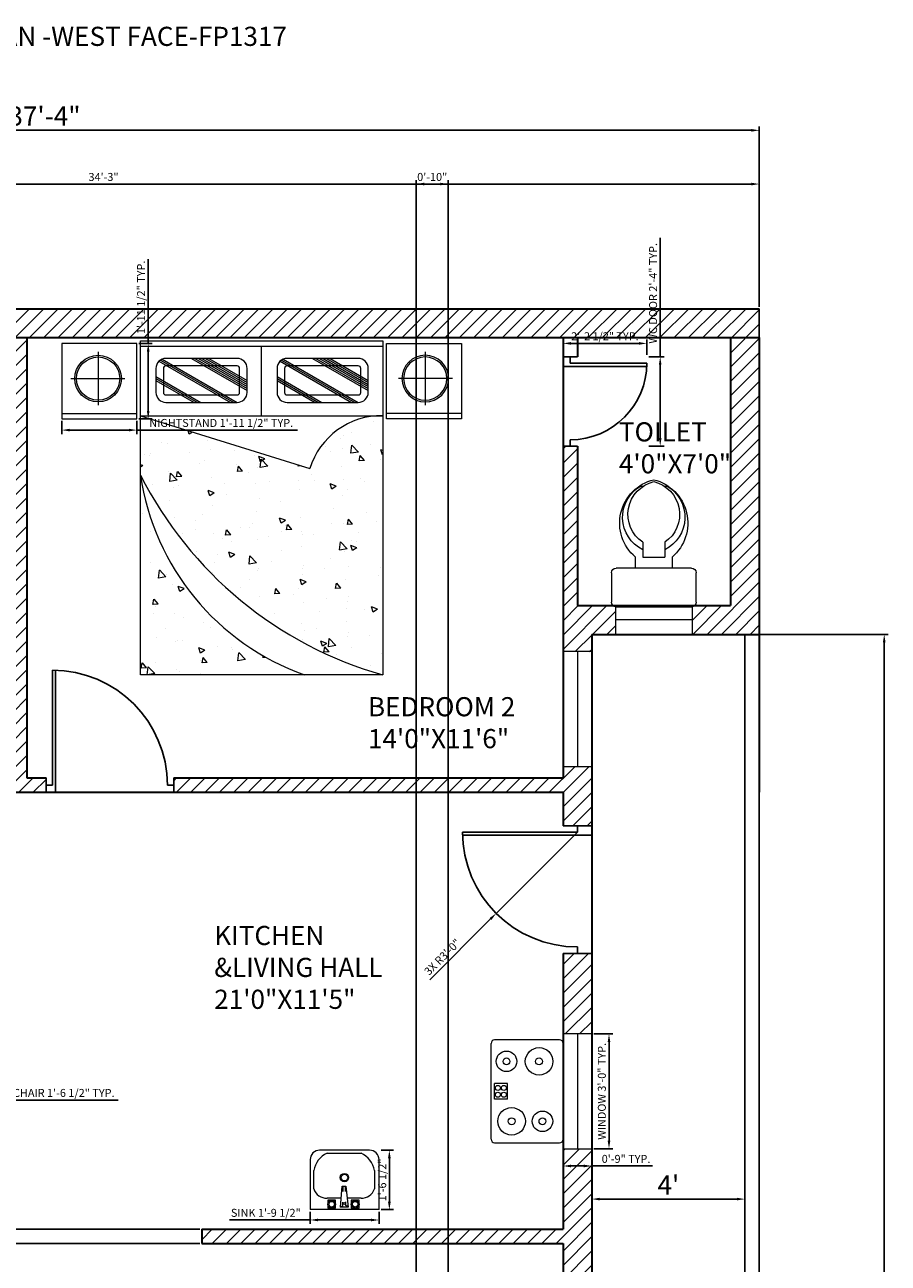
# Model space of a CAD drawing. Units: inches. Extents: x 3618 to 4156, y 1271 to 2023.
# Tile 5 of 5: x 3886 to 4156, y 1635 to 2023. Entities that reach past the tile are written whole.
import ezdxf

# ---------------------------------------------------------------- set-up
doc = ezdxf.new("R2010")
doc.units = ezdxf.units.IN
for name, color, linetype, lineweight in [('A-ANNO-DIMS', 2, 'Continuous', 18), ('A-ANNO-TITL', 7, 'Continuous', 25), ('A-AREA-IDEN', 7, 'Continuous', 18), ('A-DOOR', 4, 'Continuous', 25), ('A-EQPM', 8, 'Continuous', 18), ('A-FLOR-FIXT', 9, 'Continuous', 18), ('A-FURN', 8, 'Continuous', 18), ('A-FURN-PATT', 9, 'Continuous', 13), ('A-GLAZ', 4, 'Continuous', 18), ('A-WALL', 7, 'Continuous', 35), ('A-WALL-PATT', 252, 'Continuous', 13), ('C-PROP', 7, 'Continuous', 25)]:
    doc.layers.add(name, color=color, linetype=linetype, lineweight=lineweight)
doc.styles.get("Standard").update_dxf_attribs({"font": 'arial.ttf'})
doc.dimstyles.new('ISO-25', dxfattribs={"dimtxt": 2.5, "dimasz": 2.5, "dimexe": 1.25, "dimexo": 0.625, "dimtad": 1, "dimdec": 0, "dimlunit": 3, "dimtxsty": 'Standard', "dimcen": 2.5, "dimadec": 0, "dimazin": 0, "dimtfac": 1, "dimtdec": 0, "dimtmove": 0, "dimatfit": 3, "dimfxl": 1, "dimarcsym": 0})

# ---------------------------------------------------------------- blocks, each defined once
blk = doc.blocks.new('*D1')
at = {"layer": 'A-ANNO-DIMS', "color": 0, "lineweight": -2, "transparency": 16777216}
for p, q in [((4063.19, 1642.81), (4063.19, 1656.03)), ((4065.69, 1654.78), (4108.69, 1654.78)), ((4111.19, 1642.81), (4111.19, 1656.03))]:
    blk.add_line(p, q, dxfattribs=at)
at = {"layer": 'A-ANNO-DIMS', "color": 0, "transparency": 16777216}
for points in [[(4065.69, 1655.2), (4065.69, 1654.37), (4063.19, 1654.78)], [(4108.69, 1655.2), (4108.69, 1654.37), (4111.19, 1654.78)]]:
    blk.add_solid(points, dxfattribs=at)
at = {"layer": 'Defpoints', "color": 0, "transparency": 16777216}
for p in [(4111.19, 1654.78), (4063.19, 1642.19), (4111.19, 1642.19)]:
    blk.add_point(p, dxfattribs=at)
at = {"layer": 'A-ANNO-DIMS', "color": 0, "transparency": 16777216, "insert": (4087.19, 1658.41), "char_height": 6, "attachment_point": 5}
blk.add_mtext("4'", dxfattribs=at)
blk = doc.blocks.new('*D4')
at = {"layer": 'A-ANNO-DIMS', "color": 0, "lineweight": -2, "transparency": 16777216}
for p, q in [((3667.69, 1934.44), (3667.69, 1991.05)), ((3670.19, 1989.8), (4113.19, 1989.8)), ((4115.69, 1934.44), (4115.69, 1991.05))]:
    blk.add_line(p, q, dxfattribs=at)
at = {"layer": 'A-ANNO-DIMS', "color": 0, "transparency": 16777216}
for points in [[(3670.19, 1990.21), (3670.19, 1989.38), (3667.69, 1989.8)], [(4113.19, 1990.21), (4113.19, 1989.38), (4115.69, 1989.8)]]:
    blk.add_solid(points, dxfattribs=at)
at = {"layer": 'Defpoints', "color": 0, "transparency": 16777216}
for p in [(4115.69, 1989.8), (3667.69, 1933.81), (4115.69, 1933.81)]:
    blk.add_point(p, dxfattribs=at)
at = {"layer": 'A-ANNO-DIMS', "color": 0, "transparency": 16777216, "insert": (3891.69, 1993.49), "char_height": 6, "width": 8.5863, "attachment_point": 5}
blk.add_mtext('37\'-4"', dxfattribs=at)
blk = doc.blocks.new('A$C3A735CB7')
for p, q in [((0, 0.38), (0, 0.06)), ((0, 0.38), (0.44, 0.38)), ((0.1776, 0.3701), (0.1276, 0.3701)), ((0.1276, 0.3701), (0.1276, 0.3201)), ((0.1276, 0.3201), (0.1776, 0.3201)), ((0.1776, 0.3201), (0.1776, 0.3701)), ((0.1967, 0.364), (0.2114, 0.353)), ((0.2127, 0.229), (0.1967, 0.364)), ((0.1973, 0.3646), (0.2473, 0.3646)), ((0.2114, 0.353), (0.2127, 0.3309)), ((0.247, 0.364), (0.2311, 0.353)), ((0.2311, 0.353), (0.2311, 0.3321)), ((0.2473, 0.3646), (0.236, 0.2302)), ((0.2776, 0.3701), (0.2776, 0.3201)), ((0.3276, 0.3701), (0.2776, 0.3701)), ((0.2776, 0.3201), (0.3276, 0.3201)), ((0.3276, 0.3201), (0.3276, 0.3701)), ((0.44, 0.06), (0.44, 0.38)), ((0.0298, 0.1297), (0.0298, 0.2468)), ((0.1148, 0.3068), (0.2035, 0.3068)), ((0.2163, 0.2339), (0.2163, 0.2646)), ((0.2323, 0.2327), (0.2323, 0.2634)), ((0.2425, 0.3068), (0.3319, 0.3068)), ((0.4169, 0.2468), (0.4169, 0.1297)), ((0.2114, 0.229), (0.2163, 0.2339)), ((0.236, 0.2302), (0.2127, 0.229)), ((0.2348, 0.229), (0.2323, 0.2327)), ((0.3319, 0.0197), (0.1148, 0.0197)), ((0.06, 0), (0.38, 0))]:
    blk.add_line(p, q)
for centre, radius in [((0.1526, 0.3451), 0.025), ((0.1526, 0.3451), 0.018), ((0.2213, 0.3407), 0.00737), ((0.3026, 0.3451), 0.025), ((0.3026, 0.3451), 0.018), ((0.2215, 0.1752), 0.0272), ((0.2215, 0.1752), 0.0211)]:
    blk.add_circle(centre, radius)
for centre, radius, start, end in [((0.1116, 0.2211), 0.0858, 87.8863, 162.54889), ((0.3351, 0.2211), 0.0858, 17.45111, 92.1137), ((0.1741, 0.1534), 0.1462, 189.3166, 246.07188), ((0.2726, 0.1534), 0.1462, 293.92812, 350.6834), ((0.06, 0.06), 0.06, 180, 270), ((0.38, 0.06), 0.06, 270, 0)]:
    blk.add_arc(centre, radius, start, end)
blk = doc.blocks.new('A$C02F3725D')
for p, q in [((0.025, 0.69), (0.435, 0.69)), ((0, 0.505), (0, 0.665)), ((0.46, 0.665), (0.46, 0.505)), ((0.435, 0.48), (0.025, 0.48)), ((0.13, 0.48), (0.13, 0.42)), ((0.33, 0.42), (0.33, 0.48)), ((0.17, 0.34), (0.17, 0.42)), ((0.17, 0.42), (0.29, 0.42)), ((0.29, 0.34), (0.29, 0.42)), ((0.1578, 0.035), (0.1724, 0.035)), ((0.2876, 0.035), (0.3022, 0.035))]:
    blk.add_line(p, q)
for centre, radius, start, end in [((0.025, 0.665), 0.025, 90, 180), ((0.435, 0.665), 0.025, 0, 90), ((0.025, 0.505), 0.025, 180, 270), ((0.435, 0.505), 0.025, 270, 0), ((0.2874, 0.2356), 0.2425, 130.48854, 256.29645), ((0.1726, 0.2356), 0.2425, 283.70355, 49.51146), ((0.2568, 0.2042), 0.196, 116.27421, 239.66679), ((0.2732, 0.1883), 0.1834, 124.2157, 256.39399), ((0.1868, 0.1883), 0.1834, 283.60601, 55.7843), ((0.2032, 0.2042), 0.196, 300.33321, 63.72579)]:
    blk.add_arc(centre, radius, start, end)
blk = doc.blocks.new('DOOR-SWING-36')
for p, q in [((-1, -2.25), (-1, 36)), ((0, 0), (0, 36)), ((-38, 0), (-38, 2.25)), ((-36, 0), (-38, 0)), ((-38, 0), (-38, -2.25)), ((2, 0), (0, 0)), ((2, 2.25), (2, -2.25))]:
    blk.add_line(p, q)
blk.add_arc((0, 0), 36, 90, 180)
blk = doc.blocks.new('DOOR-SWING-24')
for p, q in [((-26, 0), (-26, 2.25)), ((-1, 2.25), (-1, -24)), ((2, -2.25), (2, 2.25)), ((-24, 0), (-26, 0)), ((-26, 0), (-26, -2.25)), ((2, 0), (0, 0)), ((0, 0), (0, -24))]:
    blk.add_line(p, q)
blk.add_arc((0, 0), 24, 180, 270)
blk = doc.blocks.new('WINDOW-24X9')
for p, q in [((0, 0), (0, 9)), ((0, 9), (24, 9)), ((24, 9), (24, 0)), ((24, 4.5), (0, 4.5)), ((24, 0), (0, 0))]:
    blk.add_line(p, q)
blk = doc.blocks.new('WINDOW-36X9')
for p, q in [((0, 36), (0, 0)), ((9, 36), (0, 36)), ((4.5, 36), (4.5, 0)), ((9, 0), (9, 36)), ((0, 0), (9, 0))]:
    blk.add_line(p, q)
blk = doc.blocks.new('NIGHTSTAND-24')
for p, q in [((0, 23.56), (0, 0)), ((23.56, 23.56), (0, 23.56)), ((23.56, 0), (23.56, 23.56)), ((11.4, 20.97), (11.4, 4.24)), ((2.83, 12.61), (19.77, 12.61)), ((0, 1.65), (23.56, 1.65)), ((0, 0), (23.56, 0))]:
    blk.add_line(p, q)
for radius in [7.3, 6.77]:
    blk.add_circle((11.4, 12.61), radius)
blk = doc.blocks.new('BED-DOUBLE')
for p, q in [((0, 0), (0, 104.72)), ((0, 104.72), (75.92, 104.72)), ((0, 103.01), (75.92, 103.01)), ((37.96, 81.21), (37.96, 103.01)), ((75.92, 104.72), (75.92, 0)), ((0, 81.21), (53.06, 64.63)), ((0, 81.21), (75.92, 81.21)), ((75.92, 0), (0, 0))]:
    blk.add_line(p, q)
for centre, radius, start, end in [((75.45, 57.8), 23.41, 88.8468, 163.0453), ((109.27, 117.79), 122.42, 206.7955, 254.1914), ((77.5, 73.85), 78.32, 188.2583, 250.5572)]:
    blk.add_arc(centre, radius, start, end)
blk = doc.blocks.new('*D26')
at = {"layer": 'A-ANNO-DIMS', "color": 0, "lineweight": -2, "transparency": 16777216}
for p, q in [((3859.81, 1687.94), (3859.81, 1684.56)), ((3862.31, 1685.81), (3875.68, 1685.81)), ((3878.18, 1687.94), (3878.18, 1684.56)), ((3878.18, 1685.81), (3914.8, 1685.81))]:
    blk.add_line(p, q, dxfattribs=at)
at = {"layer": 'A-ANNO-DIMS', "color": 0, "transparency": 16777216}
for points in [[(3862.31, 1686.23), (3862.31, 1685.39), (3859.81, 1685.81)], [(3875.68, 1686.23), (3875.68, 1685.39), (3878.18, 1685.81)]]:
    blk.add_solid(points, dxfattribs=at)
at = {"layer": 'Defpoints', "color": 0, "transparency": 16777216}
for p in [(3859.81, 1688.57), (3878.18, 1688.57), (3878.18, 1685.81)]:
    blk.add_point(p, dxfattribs=at)
at = {"layer": 'A-ANNO-DIMS', "color": 0, "transparency": 16777216, "insert": (3897.74, 1687.73), "char_height": 2.5, "attachment_point": 5}
blk.add_mtext('CHAIR 1\'-6 1/2" TYP.', dxfattribs=at)
blk = doc.blocks.new('*D28')
at = {"layer": 'A-ANNO-DIMS', "color": 0, "lineweight": -2, "transparency": 16777216}
for p, q in [((3897.09, 1898.74), (3897.09, 1894.58)), ((3920.66, 1898.74), (3920.66, 1894.58)), ((3899.59, 1895.83), (3918.16, 1895.83)), ((3920.66, 1895.83), (3970.96, 1895.83))]:
    blk.add_line(p, q, dxfattribs=at)
at = {"layer": 'A-ANNO-DIMS', "color": 0, "transparency": 16777216}
for points in [[(3899.59, 1896.25), (3899.59, 1895.42), (3897.09, 1895.83)], [(3918.16, 1896.25), (3918.16, 1895.42), (3920.66, 1895.83)]]:
    blk.add_solid(points, dxfattribs=at)
at = {"layer": 'Defpoints', "color": 0, "transparency": 16777216}
for p in [(3897.09, 1899.37), (3920.66, 1899.37), (3920.66, 1895.83)]:
    blk.add_point(p, dxfattribs=at)
at = {"layer": 'A-ANNO-DIMS', "color": 0, "transparency": 16777216, "insert": (3947.06, 1897.75), "char_height": 2.5, "attachment_point": 5}
blk.add_mtext('NIGHTSTAND 1\'-11 1/2" TYP.', dxfattribs=at)
blk = doc.blocks.new('*D29')
at = {"layer": 'A-ANNO-DIMS', "color": 0, "lineweight": -2, "transparency": 16777216}
for p, q in [((3924.19, 1922.93), (3924.19, 1949.45)), ((3921.28, 1922.93), (3925.44, 1922.93)), ((3924.19, 1901.87), (3924.19, 1920.43)), ((3921.28, 1899.37), (3925.44, 1899.37))]:
    blk.add_line(p, q, dxfattribs=at)
at = {"layer": 'A-ANNO-DIMS', "color": 0, "transparency": 16777216}
for points in [[(3923.77, 1920.43), (3924.61, 1920.43), (3924.19, 1922.93)], [(3923.77, 1901.87), (3924.61, 1901.87), (3924.19, 1899.37)]]:
    blk.add_solid(points, dxfattribs=at)
at = {"layer": 'Defpoints', "color": 0, "transparency": 16777216}
for p in [(3920.66, 1922.93), (3924.19, 1922.93), (3920.66, 1899.37)]:
    blk.add_point(p, dxfattribs=at)
at = {"layer": 'A-ANNO-DIMS', "color": 0, "transparency": 16777216, "insert": (3922.27, 1937.44), "char_height": 2.5, "attachment_point": 5, "rotation": 90}
blk.add_mtext('1\'-11 1/2" TYP.', dxfattribs=at)
blk = doc.blocks.new('*D34')
at = {"layer": 'A-ANNO-DIMS', "color": 0, "lineweight": -2, "transparency": 16777216}
for p, q in [((4084.64, 1918.81), (4084.64, 1956.14)), ((4081.06, 1918.81), (4085.89, 1918.81)), ((4084.64, 1893.31), (4084.64, 1916.31)), ((4081.06, 1890.81), (4085.89, 1890.81))]:
    blk.add_line(p, q, dxfattribs=at)
at = {"layer": 'A-ANNO-DIMS', "color": 0, "transparency": 16777216}
for points in [[(4084.22, 1916.31), (4085.05, 1916.31), (4084.64, 1918.81)], [(4084.22, 1893.31), (4085.05, 1893.31), (4084.64, 1890.81)]]:
    blk.add_solid(points, dxfattribs=at)
at = {"layer": 'Defpoints', "color": 0, "transparency": 16777216}
for p in [(4080.44, 1918.81), (4084.64, 1918.81), (4080.44, 1890.81)]:
    blk.add_point(p, dxfattribs=at)
at = {"layer": 'A-ANNO-DIMS', "color": 0, "transparency": 16777216, "insert": (4082.72, 1938.72), "char_height": 2.5, "attachment_point": 5, "rotation": 90}
blk.add_mtext('WC DOOR 2\'-4" TYP.', dxfattribs=at)
blk = doc.blocks.new('*D35')
at = {"layer": 'A-ANNO-DIMS', "color": 0, "lineweight": -2, "transparency": 16777216}
for p, q in [((4054.19, 1919.44), (4054.19, 1924.26)), ((4077.94, 1923.01), (4056.69, 1923.01)), ((4080.44, 1919.44), (4080.44, 1924.26))]:
    blk.add_line(p, q, dxfattribs=at)
at = {"layer": 'A-ANNO-DIMS', "color": 0, "transparency": 16777216}
for points in [[(4056.69, 1923.43), (4056.69, 1922.59), (4054.19, 1923.01)], [(4077.94, 1923.43), (4077.94, 1922.59), (4080.44, 1923.01)]]:
    blk.add_solid(points, dxfattribs=at)
at = {"layer": 'Defpoints', "color": 0, "transparency": 16777216}
for p in [(4054.19, 1923.01), (4054.19, 1918.81), (4080.44, 1918.81)]:
    blk.add_point(p, dxfattribs=at)
at = {"layer": 'A-ANNO-DIMS', "color": 0, "transparency": 16777216, "insert": (4067.31, 1924.93), "char_height": 2.5, "attachment_point": 5}
blk.add_mtext('2\'-2 1/2" TYP.', dxfattribs=at)
blk = doc.blocks.new('*D38')
at = {"layer": 'A-ANNO-DIMS', "color": 0, "lineweight": -2, "transparency": 16777216}
for p, q in [((4063.81, 1706.56), (4069.84, 1706.56)), ((4068.59, 1673.06), (4068.59, 1704.06)), ((4063.81, 1670.56), (4069.84, 1670.56))]:
    blk.add_line(p, q, dxfattribs=at)
at = {"layer": 'A-ANNO-DIMS', "color": 0, "transparency": 16777216}
for points in [[(4068.17, 1704.06), (4069, 1704.06), (4068.59, 1706.56)], [(4068.17, 1673.06), (4069, 1673.06), (4068.59, 1670.56)]]:
    blk.add_solid(points, dxfattribs=at)
at = {"layer": 'Defpoints', "color": 0, "transparency": 16777216}
for p in [(4063.19, 1706.56), (4068.59, 1706.56), (4063.19, 1670.56)]:
    blk.add_point(p, dxfattribs=at)
at = {"layer": 'A-ANNO-DIMS', "color": 0, "transparency": 16777216, "insert": (4066.67, 1688.56), "char_height": 2.5, "attachment_point": 5, "rotation": 90}
blk.add_mtext('WINDOW 3\'-0" TYP.', dxfattribs=at)
blk = doc.blocks.new('*D39')
at = {"layer": 'A-ANNO-DIMS', "color": 0, "lineweight": -2, "transparency": 16777216}
for p, q in [((4054.19, 1669.94), (4054.19, 1663.91)), ((4063.19, 1669.94), (4063.19, 1663.91)), ((4056.69, 1665.16), (4060.69, 1665.16)), ((4063.19, 1665.16), (4082.18, 1665.16))]:
    blk.add_line(p, q, dxfattribs=at)
at = {"layer": 'A-ANNO-DIMS', "color": 0, "transparency": 16777216}
for points in [[(4056.69, 1665.58), (4056.69, 1664.74), (4054.19, 1665.16)], [(4060.69, 1665.58), (4060.69, 1664.74), (4063.19, 1665.16)]]:
    blk.add_solid(points, dxfattribs=at)
at = {"layer": 'Defpoints', "color": 0, "transparency": 16777216}
for p in [(4054.19, 1670.56), (4063.19, 1670.56), (4063.19, 1665.16)]:
    blk.add_point(p, dxfattribs=at)
at = {"layer": 'A-ANNO-DIMS', "color": 0, "transparency": 16777216, "insert": (4073.93, 1667.06), "char_height": 2.5, "attachment_point": 5}
blk.add_mtext('0\'-9" TYP.', dxfattribs=at)
blk = doc.blocks.new('*D46')
at = {"layer": 'A-ANNO-DIMS', "color": 0, "lineweight": -2, "transparency": 16777216}
for p, q in [((3974.95, 1650.84), (3974.95, 1646.98)), ((3996.53, 1650.84), (3996.53, 1646.98)), ((3974.95, 1648.23), (3949.62, 1648.23)), ((3994.03, 1648.23), (3977.45, 1648.23))]:
    blk.add_line(p, q, dxfattribs=at)
at = {"layer": 'A-ANNO-DIMS', "color": 0, "transparency": 16777216}
for points in [[(3977.45, 1648.65), (3977.45, 1647.82), (3974.95, 1648.23)], [(3994.03, 1648.65), (3994.03, 1647.82), (3996.53, 1648.23)]]:
    blk.add_solid(points, dxfattribs=at)
at = {"layer": 'Defpoints', "color": 0, "transparency": 16777216}
for p in [(3974.95, 1651.47), (3996.53, 1651.47), (3974.95, 1648.23)]:
    blk.add_point(p, dxfattribs=at)
at = {"layer": 'A-ANNO-DIMS', "color": 0, "transparency": 16777216, "insert": (3961.04, 1650.15), "char_height": 2.5, "attachment_point": 5}
blk.add_mtext('SINK 1\'-9 1/2"', dxfattribs=at)
blk = doc.blocks.new('*D47')
at = {"layer": 'A-ANNO-DIMS', "color": 0, "lineweight": -2, "transparency": 16777216}
for p, q in [((3997.15, 1670.1), (4001.01, 1670.1)), ((3999.76, 1667.6), (3999.76, 1653.97)), ((3997.15, 1651.47), (4001.01, 1651.47))]:
    blk.add_line(p, q, dxfattribs=at)
at = {"layer": 'A-ANNO-DIMS', "color": 0, "transparency": 16777216}
for points in [[(3999.34, 1667.6), (4000.18, 1667.6), (3999.76, 1670.1)], [(3999.34, 1653.97), (4000.18, 1653.97), (3999.76, 1651.47)]]:
    blk.add_solid(points, dxfattribs=at)
at = {"layer": 'Defpoints', "color": 0, "transparency": 16777216}
for p in [(3996.53, 1670.1), (3996.53, 1651.47), (3999.76, 1651.47)]:
    blk.add_point(p, dxfattribs=at)
at = {"layer": 'A-ANNO-DIMS', "color": 0, "transparency": 16777216, "insert": (3997.84, 1660.78), "char_height": 2.5, "attachment_point": 5, "rotation": 90}
blk.add_mtext('1\'-6 1/2"', dxfattribs=at)
blk = doc.blocks.new('*D53')
at = {"layer": 'A-ANNO-DIMS', "color": 0, "lineweight": -2, "transparency": 16777216}
for p, q in [((4008.19, 1440.44), (4008.19, 1974.21)), ((4010.69, 1972.96), (4015.69, 1972.96)), ((4018.19, 1440.44), (4018.19, 1974.21))]:
    blk.add_line(p, q, dxfattribs=at)
at = {"layer": 'A-ANNO-DIMS', "color": 0, "transparency": 16777216}
for points in [[(4010.69, 1973.38), (4010.69, 1972.54), (4008.19, 1972.96)], [(4015.69, 1973.38), (4015.69, 1972.54), (4018.19, 1972.96)]]:
    blk.add_solid(points, dxfattribs=at)
at = {"layer": 'Defpoints', "color": 0, "transparency": 16777216}
for p in [(4018.19, 1972.96), (4008.19, 1439.81), (4018.19, 1439.81)]:
    blk.add_point(p, dxfattribs=at)
at = {"layer": 'A-ANNO-DIMS', "color": 0, "transparency": 16777216, "insert": (4013.19, 1974.86), "char_height": 2.5, "attachment_point": 5}
blk.add_mtext('0\'-10"', dxfattribs=at)
blk = doc.blocks.new('*D55')
at = {"layer": 'A-ANNO-DIMS', "color": 0, "lineweight": -2, "transparency": 16777216}
for p, q in [((3704.69, 1934.44), (3704.69, 1974.21)), ((3707.19, 1972.96), (4113.19, 1972.96)), ((4115.69, 1934.44), (4115.69, 1974.21))]:
    blk.add_line(p, q, dxfattribs=at)
at = {"layer": 'A-ANNO-DIMS', "color": 0, "transparency": 16777216}
for points in [[(3707.19, 1973.38), (3707.19, 1972.54), (3704.69, 1972.96)], [(4113.19, 1973.38), (4113.19, 1972.54), (4115.69, 1972.96)]]:
    blk.add_solid(points, dxfattribs=at)
at = {"layer": 'Defpoints', "color": 0, "transparency": 16777216}
for p in [(4115.69, 1972.96), (3704.69, 1933.81), (4115.69, 1933.81)]:
    blk.add_point(p, dxfattribs=at)
at = {"layer": 'A-ANNO-DIMS', "color": 0, "transparency": 16777216, "insert": (3910.19, 1974.86), "char_height": 2.5, "attachment_point": 5}
blk.add_mtext('34\'-3"', dxfattribs=at)
blk = doc.blocks.new('*D56')
at = {"layer": 'A-ANNO-DIMS', "color": 0, "lineweight": -2, "transparency": 16777216}
for p, q in [((4063.81, 1831.81), (4156.09, 1831.81)), ((4154.84, 1829.31), (4154.84, 1390.31)), ((4063.81, 1387.81), (4156.09, 1387.81))]:
    blk.add_line(p, q, dxfattribs=at)
at = {"layer": 'A-ANNO-DIMS', "color": 0, "transparency": 16777216}
for points in [[(4154.42, 1829.31), (4155.25, 1829.31), (4154.84, 1831.81)], [(4154.42, 1390.31), (4155.25, 1390.31), (4154.84, 1387.81)]]:
    blk.add_solid(points, dxfattribs=at)
at = {"layer": 'Defpoints', "color": 0, "transparency": 16777216}
for p in [(4063.19, 1831.81), (4063.19, 1387.81), (4154.84, 1387.81)]:
    blk.add_point(p, dxfattribs=at)
at = {"layer": 'A-ANNO-DIMS', "color": 0, "transparency": 16777216, "insert": (4152.94, 1609.81), "char_height": 2.5, "attachment_point": 5, "rotation": 90}
blk.add_mtext('37\'-0"', dxfattribs=at)
blk = doc.blocks.new('*D59')
at = {"layer": 'A-ANNO-DIMS', "color": 0, "lineweight": -2, "transparency": 16777216}
for p, q in [((3624.04, 1647.81), (3624.04, 1664.03)), ((3940.35, 1645.31), (3622.79, 1645.31)), ((3624.04, 1640.81), (3624.04, 1645.31)), ((3940.35, 1640.81), (3622.79, 1640.81)), ((3624.04, 1638.31), (3624.04, 1635.81))]:
    blk.add_line(p, q, dxfattribs=at)
at = {"layer": 'A-ANNO-DIMS', "color": 0, "transparency": 16777216}
for points in [[(3623.62, 1647.81), (3624.45, 1647.81), (3624.04, 1645.31)], [(3623.62, 1638.31), (3624.45, 1638.31), (3624.04, 1640.81)]]:
    blk.add_solid(points, dxfattribs=at)
at = {"layer": 'Defpoints', "color": 0, "transparency": 16777216}
for p in [(3624.04, 1645.31), (3940.98, 1645.31), (3940.98, 1640.81)]:
    blk.add_point(p, dxfattribs=at)
at = {"layer": 'A-ANNO-DIMS', "color": 0, "transparency": 16777216, "insert": (3622.12, 1657.17), "char_height": 2.5, "attachment_point": 5, "rotation": 90}
blk.add_mtext('0\'-4 1/2"', dxfattribs=at)
blk = doc.blocks.new('*D61')
at = {"layer": 'A-ANNO-DIMS', "color": 0, "lineweight": -2, "transparency": 16777216}
for p, q in [((4058.69, 1769.81), (4033.23, 1744.35)), ((4012.42, 1723.54), (4031.46, 1742.59))]:
    blk.add_line(p, q, dxfattribs=at)
at = {"layer": 'A-ANNO-DIMS', "color": 0, "transparency": 16777216}
blk.add_solid([(4031.17, 1742.88), (4031.76, 1742.29), (4033.23, 1744.35)], dxfattribs=at)
at = {"layer": 'Defpoints', "color": 0, "transparency": 16777216}
for p in [(4058.69, 1769.81), (4033.23, 1744.35)]:
    blk.add_point(p, dxfattribs=at)
at = {"layer": 'A-ANNO-DIMS', "color": 0, "transparency": 16777216, "insert": (4016.61, 1730.43), "char_height": 2.5, "attachment_point": 5, "rotation": 45.0004}
blk.add_mtext('3X R3\'-0"', dxfattribs=at)

msp = doc.modelspace()

# ---------------------------------------------------------------- hatches: boundary and pattern name
at = {"layer": 'A-FURN-PATT'}
h = msp.add_hatch(dxfattribs=at)
h.set_pattern_fill('ANSI31', color=256, scale=0.1649262, angle=105.04163, style=0)
h.paths.add_polyline_path([(3928.69, 1918.14), (3928.53, 1918.07), (3928.34, 1917.99), (3928.16, 1917.89), (3927.99, 1917.78), (3927.83, 1917.67), (3927.68, 1917.54), (3927.53, 1917.4), (3927.46, 1917.33), (3949.72, 1904.51), (3952.04, 1904.51), (3952.15, 1904.51), (3952.25, 1904.51), (3952.32, 1904.52)])
h = msp.add_hatch(dxfattribs=at)
h.set_pattern_fill('ANSI31', color=256, scale=0.1728632, angle=105.04163, style=0)
h.paths.add_polyline_path([(3943.48, 1918.32), (3937.43, 1918.32), (3955.19, 1908.09), (3955.19, 1911.57)])
h = msp.add_hatch(dxfattribs=at)
h.set_pattern_fill('ANSI31', color=256, scale=0.16490728, angle=105.04163, style=0)
h.paths.add_polyline_path([(3966.65, 1918.14), (3966.6, 1918.12), (3966.51, 1918.08), (3966.42, 1918.04), (3966.32, 1918), (3966.23, 1917.95), (3966.14, 1917.9), (3966.05, 1917.85), (3965.97, 1917.79), (3965.88, 1917.73), (3965.8, 1917.67), (3965.72, 1917.61), (3965.64, 1917.54), (3965.56, 1917.47), (3965.49, 1917.4), (3965.43, 1917.33), (3987.68, 1904.51), (3990.01, 1904.51), (3990.11, 1904.51), (3990.21, 1904.51), (3990.28, 1904.52)])
h = msp.add_hatch(dxfattribs=at)
h.set_pattern_fill('ANSI31', color=256, scale=0.17287723, angle=105.04163, style=0)
h.paths.add_polyline_path([(3981.44, 1918.32), (3975.39, 1918.32), (3993.15, 1908.09), (3993.15, 1911.57)])
h = msp.add_hatch(dxfattribs=at)
h.set_pattern_fill('ANSI31', color=256, scale=0.16490566, angle=105.04163, style=0)
h.paths.add_polyline_path([(3926.61, 1912.77), (3926.61, 1911.26), (3938.33, 1904.51), (3940.95, 1904.51)])
h = msp.add_hatch(dxfattribs=at)
h.set_pattern_fill('ANSI31', color=256, scale=0.16491056, angle=105.04163, style=0)
h.paths.add_polyline_path([(3964.57, 1912.77), (3964.57, 1911.26), (3976.29, 1904.51), (3978.91, 1904.51)])
h = msp.add_hatch(dxfattribs=at)
h.set_pattern_fill('AR-CONC', color=256, scale=0.104721, angle=360, style=0)
h.set_pattern_definition([(130, (4892.28, -4019.08), (-19.07861, -1.66916), [1.99494, -21.94434]), (185, (4892.28, -4019.08), (3.690674, 20.007695), [1.59595, -17.555474]), (79.549, (4890.69, -4019.218), (-15.388006, 18.33844), [1.69544, -18.64981]), (133.8158, (4892.28, -4013.76), (-28.38774, -4.40273), [2.99241, -32.91651]), (83.3644, (4889.914, -4014.126), (-24.86127, 25.91072), [2.54316, -27.97472]), (188.816, (4892.28, -4013.76), (-24.86131, 25.91067), [2.39393, -26.33321]), (159, (4889.62, -4015.09), (-15.877303, -10.709375), [1.99494, -21.94434]), (214, (4889.62, -4015.09), (-6.47199, 19.2884), [1.59595, -17.555474]), (108.5486, (4888.297, -4015.982), (-22.349247, 8.579066), [1.69544, -18.64981]), (142.5, (4892.28, -4019.079), (-0.3234425, 8.8547114), [0, -17.34268, 0, -17.821467, 0, -17.621972]), (172.5, (4892.28, -4019.079), (-6.99744, 10.491037), [0, -10.160896, 0, -16.943693, 0, -6.716299]), (212.5, (4898.2116, -4019.079), (-14.19922, -0.599921), [0, -6.6498, 0, -20.747379, 0, -27.530176]), (222.5, (4900.871, -4019.079), (-15.512277, 2.662695), [0, -8.64474, 0, -13.778388, 0, -19.550415])])
edge = h.paths.add_edge_path()
edge.add_ellipse((3997.24, 1876.92), major_axis=(16.55, -16.55), ratio=1, start_angle=136.1532, end_angle=208.0453, ccw=False)
edge.add_line((3996.77, 1900.33), (3997.71, 1900.33))
edge.add_line((3997.71, 1900.33), (3997.71, 1819.12))
edge.add_ellipse((4031.06, 1936.91), major_axis=(86.56, -86.56), ratio=1, start_angle=251.7955, end_angle=299.1914, ccw=False)
edge.add_line((3921.79, 1881.72), (3921.79, 1900.33))
edge.add_line((3921.79, 1900.33), (3974.84, 1883.75))
edge = h.paths.add_edge_path()
edge.add_line((3973.22, 1819.12), (3921.79, 1819.12))
edge.add_line((3921.79, 1819.12), (3921.79, 1881.72))
edge.add_ellipse((3999.29, 1892.97), major_axis=(-55.38, -55.38), ratio=1, start_angle=323.2583, end_angle=385.5572)
at = {"layer": 'A-WALL-PATT'}
h = msp.add_hatch(dxfattribs=at)
h.set_pattern_fill('ANSI31', color=256)
h.paths.add_polyline_path([(4115.69, 1933.81), (3704.69, 1933.81), (3704.69, 1885.81), (3713.69, 1885.81), (3713.69, 1924.81), (4115.69, 1924.81)])
h.paths.add_polyline_path([(3886.19, 1924.81), (3881.69, 1924.81), (3881.69, 1786.81), (3875.69, 1786.81), (3875.69, 1782.31), (3892.19, 1782.31), (3892.19, 1786.81), (3886.19, 1786.81)])
h.paths.add_polyline_path([(3763.69, 1784.56), (3763.69, 1786.81), (3713.69, 1786.81), (3713.69, 1782.31), (3763.69, 1782.31)], flags=17)
h.paths.add_polyline_path([(3713.69, 1825.81), (3704.69, 1825.81), (3704.69, 1764.31), (3713.69, 1764.31)])
h.paths.add_polyline_path([(3802.19, 1782.31), (3835.69, 1782.31), (3835.69, 1784.56), (3835.69, 1786.81), (3791.69, 1786.81), (3791.69, 1782.31), (3797.69, 1782.31), (3797.69, 1722.31), (3713.69, 1722.31), (3713.69, 1717.81), (3797.69, 1717.81), (3797.69, 1657.81), (3791.69, 1657.81), (3791.69, 1653.31), (3851.69, 1653.31), (3851.69, 1647.31), (3856.19, 1647.31), (3856.19, 1657.81), (3802.19, 1657.81)])
h.paths.add_polyline_path([(3713.69, 1740.31), (3704.69, 1740.31), (3704.69, 1699.81), (3713.69, 1699.81)])
h.paths.add_polyline_path([(3713.69, 1675.81), (3704.69, 1675.81), (3704.69, 1623.31), (3713.69, 1623.31)])
h.paths.add_polyline_path([(3743.18, 1533.31), (3713.69, 1533.31), (3713.69, 1563.31), (3704.69, 1563.31), (3704.69, 1524.31), (3743.18, 1524.31)])
h.paths.add_polyline_path([(3856.19, 1533.31), (3803.18, 1533.31), (3803.18, 1524.31), (3847.19, 1524.31), (3847.19, 1518.31), (3856.19, 1518.31)])
h.paths.add_polyline_path([(3856.19, 1607.31), (3853.94, 1607.31), (3851.69, 1607.31), (3851.69, 1533.31), (3856.19, 1533.31)])
h.paths.add_polyline_path([(3763.69, 1655.56), (3763.69, 1657.81), (3713.69, 1657.81), (3713.69, 1653.31), (3763.69, 1653.31)], flags=17)
h.paths.add_polyline_path([(4063.19, 1670.56), (4054.19, 1670.56), (4054.19, 1645.31), (3940.98, 1645.31), (3940.98, 1640.81), (4054.19, 1640.81), (4054.19, 1592.81), (4063.19, 1592.81)])
h.paths.add_polyline_path([(4063.19, 1532.81), (4054.19, 1532.81), (4054.19, 1454.31), (4063.19, 1454.31)])
h.paths.add_polyline_path([(4054.19, 1484.81), (3985.19, 1484.81), (3985.19, 1475.81), (4054.19, 1475.81)])
h.paths.add_polyline_path([(3925.19, 1484.81), (3856.19, 1484.81), (3856.19, 1490.81), (3847.19, 1490.81), (3847.19, 1475.81), (3925.19, 1475.81)])
h.paths.add_polyline_path([(4063.19, 1396.81), (3928.19, 1396.81), (3928.19, 1387.81), (4063.19, 1387.81)])
h.paths.add_polyline_path([(4063.19, 1418.31), (4054.19, 1418.31), (4054.19, 1396.81), (4063.19, 1396.81)])
h.paths.add_polyline_path([(4063.19, 1790.42), (4054.19, 1790.42), (4054.19, 1786.81), (3932.19, 1786.81), (3932.19, 1784.56), (3932.19, 1782.31), (4054.19, 1782.31), (4054.19, 1771.81), (4063.19, 1771.81)])
h.paths.add_polyline_path([(4070.69, 1840.81), (4058.69, 1840.81), (4058.69, 1890.81), (4056.44, 1890.81), (4054.19, 1890.81), (4054.19, 1826.42), (4063.19, 1826.42), (4063.19, 1831.81), (4070.69, 1831.81)])
h.paths.add_polyline_path([(4115.69, 1924.81), (4106.69, 1924.81), (4106.69, 1840.81), (4094.69, 1840.81), (4094.69, 1831.81), (4115.69, 1831.81)])
h.paths.add_polyline_path([(4063.19, 1731.81), (4058.69, 1731.81), (4054.19, 1731.81), (4054.19, 1706.56), (4063.19, 1706.56)])

# ---------------------------------------------------------------- linework, layer by layer
at = {"layer": 'A-DOOR'}
for p, q in [((4063.19, 1771.81), (4054.19, 1771.81)), ((4058.69, 1771.81), (4058.69, 1769.81)), ((4058.69, 1769.81), (4022.69, 1769.81)), ((4063.19, 1768.81), (4022.69, 1768.81)), ((4058.69, 1731.81), (4054.19, 1731.81)), ((4058.69, 1733.81), (4058.69, 1731.81)), ((4058.69, 1731.81), (4063.19, 1731.81))]:
    msp.add_line(p, q, dxfattribs=at)
msp.add_arc((4058.69, 1769.81), 36, 180, 270, dxfattribs=at)
at = {"layer": 'A-EQPM'}
for p, q in [((4053.11, 1704.67), (4032.71, 1704.67)), ((4031.63, 1673.52), (4031.63, 1703.6)), ((4054.19, 1673.52), (4054.19, 1703.6)), ((4032.71, 1686.14), (4032.71, 1690.98)), ((4036.73, 1690.98), (4032.71, 1690.98)), ((4036.73, 1686.14), (4036.73, 1690.98)), ((4036.73, 1686.14), (4032.71, 1686.14)), ((4032.71, 1672.45), (4053.11, 1672.45))]:
    msp.add_line(p, q, dxfattribs=at)
for centre, radius in [((4036.47, 1697.96), 3.22), ((4046.67, 1697.96), 4.3), ((4036.47, 1697.96), 1.07), ((4046.67, 1697.96), 1.07), ((4033.78, 1689.63), 0.806), ((4035.66, 1689.63), 0.806), ((4033.78, 1687.49), 0.806), ((4035.66, 1687.49), 0.806), ((4038.08, 1679.16), 4.3), ((4047.74, 1679.16), 3.22), ((4038.08, 1679.16), 1.07), ((4047.74, 1679.16), 1.07)]:
    msp.add_circle(centre, radius, dxfattribs=at)
for centre, start, end in [((4032.71, 1703.6), 90, 180), ((4053.11, 1703.6), 0.0001, 90.0001), ((4032.71, 1673.52), 180, 270), ((4053.11, 1673.52), 270, 0)]:
    msp.add_arc(centre, 1.07, start, end, dxfattribs=at)
at = {"layer": 'A-FURN'}
for points in [[(3952.04, 1918.32), (3929.75, 1918.32, 0.414214), (3926.61, 1915.18), (3926.61, 1907.65, 0.414214), (3929.75, 1904.51), (3952.04, 1904.51, 0.414214), (3955.19, 1907.65), (3955.19, 1915.18, 0.414214)], [(3990.01, 1918.32), (3967.71, 1918.32, 0.414214), (3964.57, 1915.18), (3964.57, 1907.65, 0.414214), (3967.71, 1904.51), (3990.01, 1904.51, 0.414214), (3993.15, 1907.65), (3993.15, 1915.18, 0.414214)], [(3952.04, 1915.96), (3929.75, 1915.96, 0.414214), (3928.96, 1915.18), (3928.96, 1907.65, 0.414214), (3929.75, 1906.86), (3952.04, 1906.86, 0.414214), (3952.83, 1907.65), (3952.83, 1915.18, 0.414214)], [(3990.01, 1915.96), (3967.71, 1915.96, 0.414214), (3966.93, 1915.18), (3966.93, 1907.65, 0.414214), (3967.71, 1906.86), (3990.01, 1906.86, 0.414214), (3990.79, 1907.65), (3990.79, 1915.18, 0.414214)]]:
    msp.add_lwpolyline(points, format="xyb", close=True, dxfattribs=at)
at = {"layer": 'A-WALL'}
for p, q in [((3704.69, 1933.81), (4115.69, 1933.81)), ((3713.69, 1924.81), (4115.69, 1924.81)), ((3886.19, 1924.81), (3886.19, 1786.81)), ((4054.19, 1924.81), (4054.19, 1786.81)), ((4058.69, 1924.81), (4058.69, 1918.81)), ((4106.69, 1924.81), (4106.69, 1840.81)), ((4115.69, 1924.81), (4115.69, 1782.31)), ((4058.69, 1890.81), (4058.69, 1840.81)), ((4058.69, 1840.81), (4106.69, 1840.81)), ((4063.19, 1831.81), (4063.19, 1387.81)), ((4063.19, 1831.81), (4115.69, 1831.81)), ((3886.19, 1786.81), (3892.19, 1786.81)), ((3932.19, 1786.81), (4054.19, 1786.81)), ((3802.19, 1782.31), (4054.19, 1782.31)), ((4054.19, 1782.31), (4054.19, 1771.81)), ((4054.19, 1731.81), (4054.19, 1645.31)), ((3940.98, 1645.31), (3940.98, 1640.81)), ((3940.98, 1645.31), (4054.19, 1645.31)), ((3940.98, 1640.81), (4054.19, 1640.81)), ((4054.19, 1640.81), (4054.19, 1396.81))]:
    msp.add_line(p, q, dxfattribs=at)
at = {"layer": 'C-PROP'}
for p, q in [((4115.69, 1933.81), (4115.69, 1341.81)), ((4111.19, 1831.81), (4111.19, 1341.81))]:
    msp.add_line(p, q, dxfattribs=at)

# ---------------------------------------------------------------- block references
at = {"layer": 'A-DOOR', "rotation": 89.99999999999972}
msp.add_blockref('DOOR-SWING-24', (4056.44, 1916.81), dxfattribs=at)
at = {"layer": 'A-DOOR', "extrusion": (0, 0, -1), "zscale": -1}
msp.add_blockref('DOOR-SWING-36', (-3894.19, 1784.56), dxfattribs=at)
at = {"layer": 'A-FLOR-FIXT', "rotation": 180}
for name, p, xscale, yscale, zscale in [('A$C02F3725D', (4069.35, 1880.26), -57.66831845044013, 57.66831845044013, 57.66831845044013), ('A$C3A735CB7', (3996.53, 1670.1), 49.02550333380638, 49.02550333380638, 49.02550333380638)]:
    msp.add_blockref(name, p, dxfattribs=dict(at, xscale=xscale, yscale=yscale, zscale=zscale))
at = {"layer": 'A-FURN'}
for name, p in [('NIGHTSTAND-24', (3897.09, 1899.37)), ('BED-DOUBLE', (3921.78, 1819.12))]:
    msp.add_blockref(name, p, dxfattribs=at)
at = {"layer": 'A-FURN', "extrusion": (0, 0, -1), "zscale": -1}
msp.add_blockref('NIGHTSTAND-24', (-4022.4, 1899.37), dxfattribs=at)
at = {"layer": 'A-GLAZ'}
for name, p in [('WINDOW-24X9', (4070.69, 1831.81)), ('WINDOW-36X9', (4054.19, 1790.42)), ('WINDOW-36X9', (4054.19, 1670.56))]:
    msp.add_blockref(name, p, dxfattribs=at)

# ---------------------------------------------------------------- texts
at = {"layer": 'A-ANNO-TITL', "insert": (3776.07, 2022.26), "char_height": 6, "attachment_point": 1}
msp.add_mtext('38X50\\{1900sq ft\\}HOUSE PLAN -WEST FACE-FP1317', dxfattribs=at)
at = {"layer": 'A-AREA-IDEN', "char_height": 6, "attachment_point": 1}
for s, insert in [('TOILET\\P4\'0"X7\'0"', (4071.69, 1898.28)), ('BEDROOM 2\\P14\'0"X11\'6"', (3993.05, 1812.12)), ('KITCHEN\\P&LIVING HALL\\P21\'0"X11\'5"', (3944.88, 1740.41))]:
    msp.add_mtext(s, dxfattribs=dict(at, insert=insert))

# ---------------------------------------------------------------- dimensions: what is measured, and where the dimension line sits
at = {"layer": 'A-ANNO-DIMS'}
for base, p1, p2, override, picture, middle in [((4115.69, 1989.8), (3667.69, 1933.81), (4115.69, 1933.81), {"dimtxt": 6, "dimclrd": 0, "dimclre": 0, "dimclrt": 0}, '*D4', (3891.69, 1993.49)), ((4115.69, 1972.96), (3704.69, 1933.81), (4115.69, 1933.81), {"dimdec": 1, "dimlfac": 1, "dimrnd": 0, "dimzin": 1, "dimdsep": 46, "dimlunit": 4, "dimfrac": 2}, '*D55', (3910.19, 1974.86)), ((4018.19, 1972.96), (4008.19, 1439.81), (4018.19, 1439.81), {"dimdec": 1, "dimlfac": 1, "dimrnd": 0, "dimzin": 1, "dimdsep": 46, "dimlunit": 4, "dimfrac": 2}, '*D53', (4013.19, 1974.86)), ((4111.19, 1654.78), (4063.19, 1642.19), (4111.19, 1642.19), {"dimtxt": 6, "dimclrd": 0, "dimclre": 0, "dimclrt": 0}, '*D1', (4087.19, 1658.41))]:
    dim = msp.add_linear_dim(base=base, p1=p1, p2=p2, dimstyle='ISO-25', override=override, dxfattribs=at)
    dim.commit()
    dim.dimension.update_dxf_attribs({"geometry": picture, "text_midpoint": middle})
for base, p1, p2, angle, text, picture, middle in [((4084.64, 1918.81), (4080.44, 1890.81), (4080.44, 1918.81), 90, 'WC DOOR <> TYP.', '*D34', (4082.72, 1938.72)), ((3924.19, 1922.93), (3920.66, 1899.37), (3920.66, 1922.93), 90, '<> TYP.', '*D29', (3922.27, 1937.44)), ((4054.18781808, 1923.01015181), (4080.43781808, 1918.81015181), (4054.18781808, 1918.81015181), 180, '<> TYP.', '*D35', (4067.31281808, 1924.92778483)), ((4068.59, 1706.56), (4063.19, 1670.56), (4063.19, 1706.56), 90, 'WINDOW <> TYP.', '*D38', (4066.67, 1688.56)), ((3974.95, 1648.23), (3996.53, 1651.47), (3974.95, 1651.47), 180, 'SINK <>', '*D46', (3961.04, 1650.15))]:
    dim = msp.add_linear_dim(base=base, p1=p1, p2=p2, angle=angle, text=text, dimstyle='ISO-25', override={"dimdec": 1, "dimlfac": 1, "dimrnd": 0, "dimzin": 1, "dimdsep": 46, "dimlunit": 4, "dimfrac": 2}, dxfattribs=at)
    dim.commit()
    dim.dimension.update_dxf_attribs({"geometry": picture, "text_midpoint": middle})
for base, p1, p2, text, picture, middle in [((3920.66, 1895.83), (3897.09, 1899.37), (3920.66, 1899.37), 'NIGHTSTAND <> TYP.', '*D28', (3947.06, 1897.75)), ((3878.18, 1685.81), (3859.81, 1688.57), (3878.18, 1688.57), 'CHAIR <> TYP.', '*D26', (3897.74, 1687.73)), ((4063.19, 1665.16), (4054.19, 1670.56), (4063.19, 1670.56), '<> TYP.', '*D39', (4073.93, 1667.06))]:
    dim = msp.add_linear_dim(base=base, p1=p1, p2=p2, text=text, dimstyle='ISO-25', override={"dimdec": 1, "dimlfac": 1, "dimrnd": 0, "dimzin": 1, "dimdsep": 46, "dimlunit": 4, "dimfrac": 2}, dxfattribs=at)
    dim.commit()
    dim.dimension.update_dxf_attribs({"geometry": picture, "text_midpoint": middle})
for base, p1, p2, angle, picture, middle in [((4154.84, 1387.81), (4063.19, 1831.81), (4063.19, 1387.81), 90, '*D56', (4152.94, 1609.81)), ((3999.76, 1651.47), (3996.53, 1670.1), (3996.53, 1651.47), 270, '*D47', (3997.84, 1660.78)), ((3624.04, 1645.31), (3940.98, 1640.81), (3940.98, 1645.31), 90, '*D59', (3622.12, 1657.17))]:
    dim = msp.add_linear_dim(base=base, p1=p1, p2=p2, angle=angle, dimstyle='ISO-25', override={"dimdec": 1, "dimlfac": 1, "dimrnd": 0, "dimzin": 1, "dimdsep": 46, "dimlunit": 4, "dimfrac": 2}, dxfattribs=at)
    dim.commit()
    dim.dimension.update_dxf_attribs({"geometry": picture, "text_midpoint": middle})
dim = msp.add_radius_dim(center=(4058.69, 1769.81), mpoint=(4033.23, 1744.35), text='3X <>', dimstyle='ISO-25', override={"dimdec": 1, "dimlfac": 1, "dimrnd": 0, "dimzin": 1, "dimdsep": 46, "dimlunit": 4, "dimfrac": 2}, dxfattribs=at)
dim.commit()
dim.dimension.update_dxf_attribs({"geometry": '*D61', "text_midpoint": (4017.96, 1729.08), "dimtype": 164})

doc.saveas('drawing.dxf')
